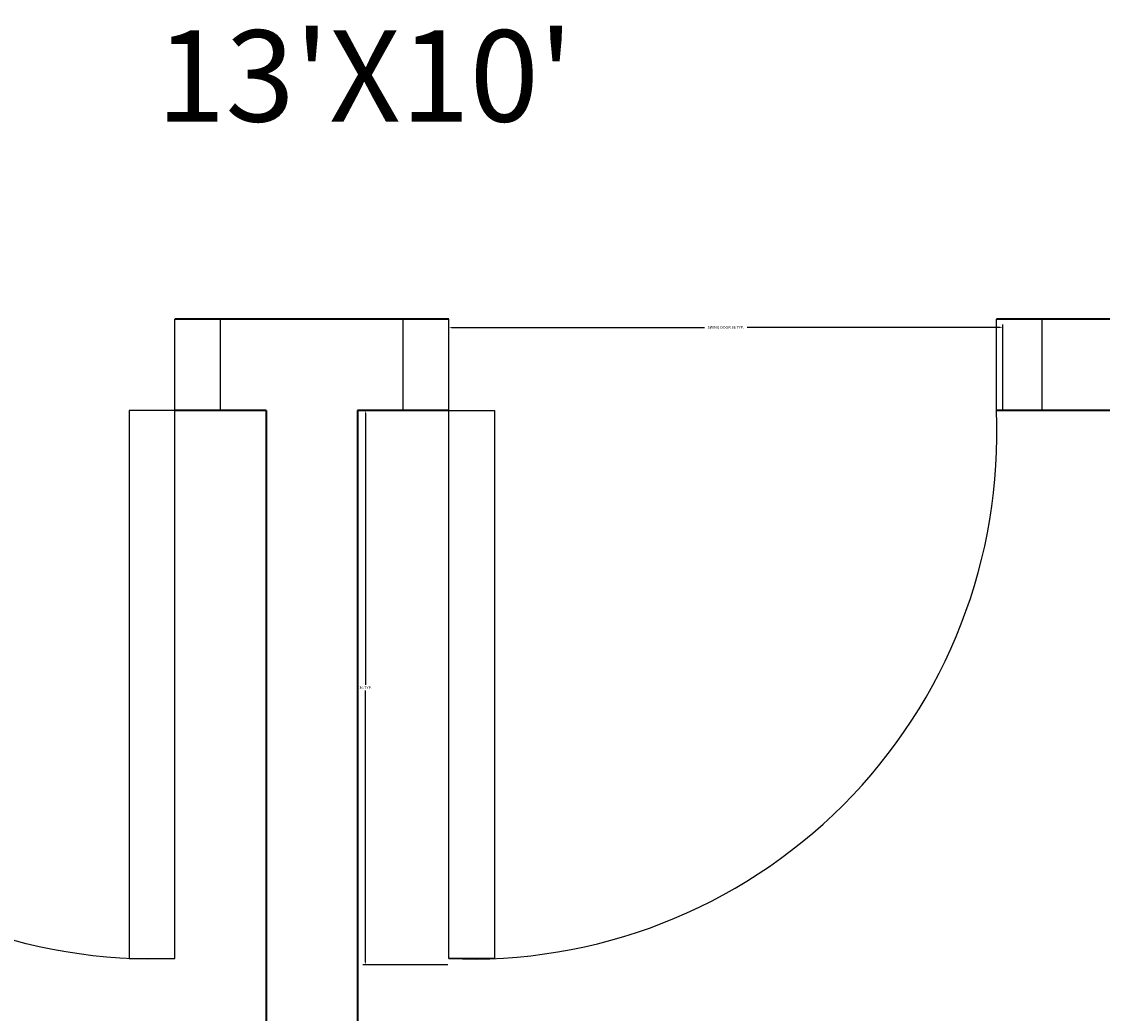
# Model space of a CAD drawing. Units: inches. Extents: x 4159 to 4826, y 299 to 1026.
# Tile 18 of 37: x 4305 to 4376, y 494 to 559. Entities that reach past the tile are written whole.
import ezdxf

# ---------------------------------------------------------------- set-up
doc = ezdxf.new("R2010")
doc.units = ezdxf.units.IN
for name, color, linetype, lineweight in [('A-ANNO-DIMS', 2, 'Continuous', 18), ('A-AREA-IDEN', 7, 'Continuous', 18), ('A-DOOR', 4, 'Continuous', 25), ('A-WALL', 7, 'Continuous', 35)]:
    doc.layers.add(name, color=color, linetype=linetype, lineweight=lineweight)
doc.styles.get("Standard").update_dxf_attribs({"font": 'arial.ttf'})
doc.dimstyles.get("Standard").update_dxf_attribs({"dimtxt": 0.18, "dimasz": 0.18, "dimexe": 0.18, "dimexo": 0.0625, "dimgap": 0.09, "dimtad": 0, "dimtih": 1, "dimtoh": 1, "dimdec": 4, "dimzin": 0, "dimdsep": 46, "dimtxsty": 'Standard', "dimcen": 0.09, "dimadec": 0, "dimazin": 0, "dimtfac": 1, "dimtdec": 4, "dimtofl": 0, "dimtmove": 0, "dimatfit": 3, "dimfxl": 1, "dimtolj": 1, "dimtzin": 0, "dimarcsym": 0})

# ---------------------------------------------------------------- blocks, each defined once
blk = doc.blocks.new('DOOR-SWING-36IN')
blk.add_lwpolyline([(0, 0), (-3, 0), (-3, 36), (0, 36)], close=True)
blk.add_arc((-1.5, 1.5), 34.533, 87.51045, 182.48955)
blk = doc.blocks.new('DOOR-FRAME-36IN')
for p, q in [((0, 6), (0, 0)), ((3, 6), (3, 0)), ((39, 6), (39, 0)), ((42, 6), (42, 0))]:
    blk.add_line(p, q)
blk = doc.blocks.new('*D17')
at = {"layer": 'A-ANNO-DIMS', "color": 0, "lineweight": -2, "transparency": 16777216}
for p, q in [((4333.31, 533.317), (4333.31, 538.897)), ((4333.49, 538.717), (4350.12, 538.717)), ((4369.551, 538.717), (4352.921, 538.717)), ((4369.731, 533.317), (4369.731, 538.897))]:
    blk.add_line(p, q, dxfattribs=at)
at = {"layer": 'A-ANNO-DIMS', "color": 0, "transparency": 16777216}
for points in [[(4333.49, 538.747), (4333.49, 538.687), (4333.31, 538.717)], [(4369.551, 538.747), (4369.551, 538.687), (4369.731, 538.717)]]:
    blk.add_solid(points, dxfattribs=at)
at = {"layer": 'Defpoints', "color": 0, "transparency": 16777216}
for p in [(4333.31, 538.717), (4333.31, 533.254), (4369.731, 533.254)]:
    blk.add_point(p, dxfattribs=at)
at = {"layer": 'A-ANNO-DIMS', "color": 0, "transparency": 16777216, "insert": (4351.521, 538.717), "char_height": 0.18, "attachment_point": 5}
blk.add_mtext('\\A1;SWING DOOR 36 TYP.', dxfattribs=at)
blk = doc.blocks.new('*D18')
at = {"layer": 'A-ANNO-DIMS', "color": 0, "lineweight": -2, "transparency": 16777216}
for p, q in [((4333.248, 533.254), (4327.667, 533.254)), ((4327.847, 533.074), (4327.847, 515.226)), ((4327.847, 497.014), (4327.847, 514.862)), ((4333.248, 496.834), (4327.667, 496.834))]:
    blk.add_line(p, q, dxfattribs=at)
at = {"layer": 'A-ANNO-DIMS', "color": 0, "transparency": 16777216}
for points in [[(4327.817, 533.074), (4327.877, 533.074), (4327.847, 533.254)], [(4327.817, 497.014), (4327.877, 497.014), (4327.847, 496.834)]]:
    blk.add_solid(points, dxfattribs=at)
at = {"layer": 'Defpoints', "color": 0, "transparency": 16777216}
for p in [(4333.31, 533.254), (4327.847, 496.834), (4333.31, 496.834)]:
    blk.add_point(p, dxfattribs=at)
at = {"layer": 'A-ANNO-DIMS', "color": 0, "transparency": 16777216, "insert": (4327.847, 515.044), "char_height": 0.18, "attachment_point": 5}
blk.add_mtext('\\A1;36 TYP.', dxfattribs=at)
blk = doc.blocks.new('*D44')
at = {"layer": 'A-ANNO-DIMS', "color": 0, "lineweight": -2, "transparency": 16777216}
for p, q in [((4287.263, 963.093), (4158.88, 963.093)), ((4159.06, 962.913), (4159.06, 647.826)), ((4159.06, 332.375), (4159.06, 647.462)), ((4447.248, 332.195), (4158.88, 332.195))]:
    blk.add_line(p, q, dxfattribs=at)
at = {"layer": 'A-ANNO-DIMS', "color": 0, "transparency": 16777216}
for points in [[(4159.03, 962.913), (4159.09, 962.913), (4159.06, 963.093)], [(4159.03, 332.375), (4159.09, 332.375), (4159.06, 332.195)]]:
    blk.add_solid(points, dxfattribs=at)
at = {"layer": 'Defpoints', "color": 0, "transparency": 16777216}
for p in [(4287.326, 963.093), (4159.06, 332.195), (4447.31, 332.195)]:
    blk.add_point(p, dxfattribs=at)
at = {"layer": 'A-ANNO-DIMS', "color": 0, "transparency": 16777216, "insert": (4159.06, 647.644), "char_height": 0.18, "attachment_point": 5}
blk.add_mtext('\\A1;630.9', dxfattribs=at)

msp = doc.modelspace()

# ---------------------------------------------------------------- linework, layer by layer
at = {"layer": 'A-DOOR'}
for p, q in [((4315.31, 533.254), (4315.31, 539.254)), ((4318.31, 533.254), (4318.31, 539.254))]:
    msp.add_line(p, q, dxfattribs=at)
at = {"layer": 'A-WALL'}
for p, q in [((4333.31, 539.254), (4315.31, 539.254)), ((4447.31, 539.254), (4369.31, 539.254)), ((4321.31, 533.254), (4315.31, 533.254)), ((4321.31, 533.254), (4321.31, 401.254)), ((4327.31, 533.254), (4327.31, 401.254)), ((4333.31, 533.254), (4327.31, 533.254)), ((4447.31, 533.254), (4369.31, 533.254))]:
    msp.add_line(p, q, dxfattribs=at)

# ---------------------------------------------------------------- block references
at = {"layer": 'A-DOOR', "rotation": 180}
for name, p in [('DOOR-FRAME-36IN', (4372.31, 539.254)), ('DOOR-SWING-36IN', (4333.31, 533.254))]:
    msp.add_blockref(name, p, dxfattribs=at)
at = {"layer": 'A-DOOR', "extrusion": (0, 0, -1), "zscale": -1, "rotation": 180}
msp.add_blockref('DOOR-SWING-36IN', (-4315.31, 533.254), dxfattribs=at)

# ---------------------------------------------------------------- texts
at = {"layer": 'A-AREA-IDEN'}
msp.add_text("13'X10'", height=6, dxfattribs=at).set_placement((4314.093, 552.235))

# ---------------------------------------------------------------- dimensions: what is measured, and where the dimension line sits
at = {"layer": 'A-ANNO-DIMS'}
dim = msp.add_linear_dim(base=(4159.06, 332.195), p1=(4287.326, 963.093), p2=(4447.31, 332.195), angle=90, dimstyle='Standard', override={"dimdec": 1, "dimlfac": 1, "dimrnd": 0, "dimzin": 0, "dimdsep": 46, "dimlunit": 2}, dxfattribs=at)
dim.commit()
dim.dimension.update_dxf_attribs({"geometry": '*D44', "text_midpoint": (4159.06, 647.644)})
for base, p1, p2, angle, text, picture, middle in [((4333.31, 538.717), (4369.731, 533.254), (4333.31, 533.254), 180, 'SWING DOOR <> TYP.', '*D17', (4351.521, 538.717)), ((4327.847, 496.834), (4333.31, 533.254), (4333.31, 496.834), 270, '<> TYP.', '*D18', (4327.847, 515.044))]:
    dim = msp.add_linear_dim(base=base, p1=p1, p2=p2, angle=angle, text=text, dimstyle='Standard', override={"dimdec": 0, "dimlfac": 1, "dimrnd": 0, "dimzin": 0, "dimdsep": 46, "dimlunit": 2}, dxfattribs=at)
    dim.commit()
    dim.dimension.update_dxf_attribs({"geometry": picture, "text_midpoint": middle})

doc.saveas('drawing.dxf')
